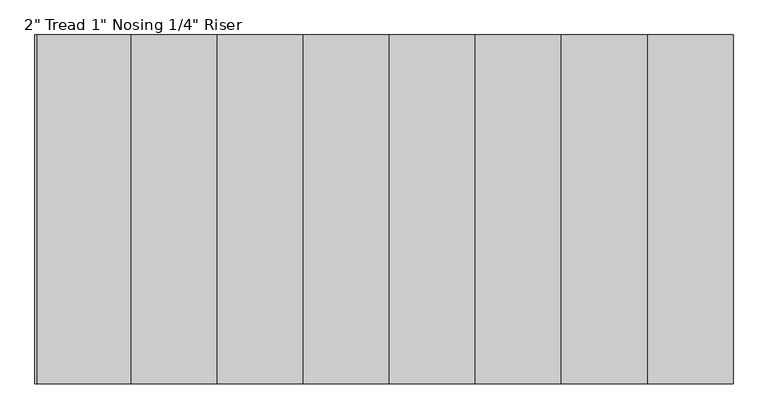
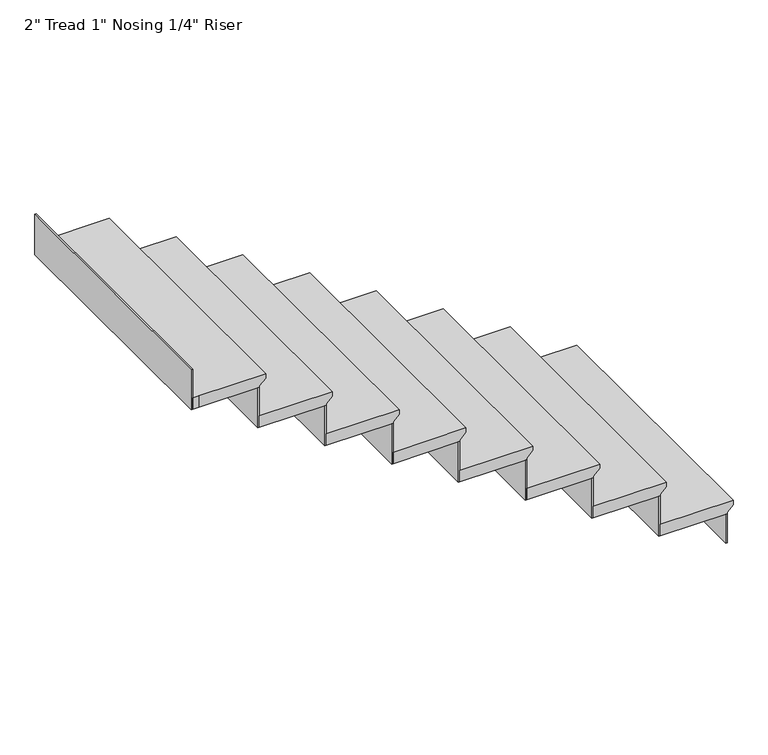
"""IFC4 building model written with IfcOpenShell, lengths in millimetres: stair flight geometry."""

from ifc_helpers import new_model, si_unit, origin, place, context, project, spatial, faceted_brep, source, transform, mapped, element, save


def stair_flight_1352b5f3(model_context):
    return source(origin(), model_context, "Body", "Brep", [
        faceted_brep([(-7986.2683044, -2706.1923176, 158.75), (-7986.2683044, -2706.1923176, 177.8), (-7986.2683044, -3838.3891189, 177.8), (-7986.2683044, -3838.3891189, 158.75), (-8011.6683044, -2706.1923176, 133.35), (-8011.6683044, -3838.3891189, 133.35), (-8291.0683044, -2706.1923176, 177.8), (-8291.0683044, -3838.3891189, 177.8), (-8011.6683044, -3838.3891189, 127.0), (-8291.0683044, -3838.3891189, 127.0), (-8291.0683044, -2706.1923176, 127.0), (-8011.6683044, -2706.1923176, 127.0)], [[[0, 1, 2, 3]], [[4, 0, 3, 5]], [[2, 1, 6, 7]], [[8, 9, 10, 11]], [[2, 7, 9, 8, 5, 3]], [[8, 11, 4, 5]], [[6, 1, 0, 4, 11, 10]], [[7, 6, 10, 9]]]),
        faceted_brep([(-8011.6683044, -2706.1923176, 127.0), (-8011.6683044, -2706.1923176, 0.0), (-8018.0183044, -2706.1923176, 0.0), (-8018.0183044, -2706.1923176, 127.0), (-8011.6683044, -3838.3891189, 127.0), (-8018.0183044, -3838.3891189, 127.0), (-8018.0183044, -3838.3891189, 0.0), (-8011.6683044, -3838.3891189, 0.0)], [[[0, 1, 2, 3]], [[4, 5, 6, 7]], [[1, 0, 4, 7]], [[2, 1, 7, 6]], [[3, 2, 6, 5]], [[0, 3, 5, 4]]]),
        faceted_brep([(-8291.0683044, -2706.1923176, 304.8), (-8291.0683044, -2706.1923176, 127.0), (-8297.4183044, -2706.1923176, 127.0), (-8297.4183044, -2706.1923176, 304.8), (-8291.0683044, -3838.3891189, 304.8), (-8297.4183044, -3838.3891189, 304.8), (-8297.4183044, -3838.3891189, 127.0), (-8291.0683044, -3838.3891189, 127.0)], [[[0, 1, 2, 3]], [[4, 5, 6, 7]], [[1, 0, 4, 7]], [[2, 1, 7, 6]], [[3, 2, 6, 5]], [[0, 3, 5, 4]]]),
        faceted_brep([(-8265.6683044, -3838.3891189, 355.6), (-8265.6683044, -2706.1923176, 355.6), (-8570.4683044, -2706.1923176, 355.6), (-8570.4683044, -3838.3891189, 355.6), (-8291.0683044, -3838.3891189, 304.8), (-8570.4683044, -3838.3891189, 304.8), (-8570.4683044, -2706.1923176, 304.8), (-8291.0683044, -2706.1923176, 304.8), (-8291.0683044, -3838.3891189, 311.15), (-8265.6683044, -3838.3891189, 336.55), (-8291.0683044, -2706.1923176, 311.15), (-8265.6683044, -2706.1923176, 336.55)], [[[0, 1, 2, 3]], [[4, 5, 6, 7]], [[0, 3, 5, 4, 8, 9]], [[4, 7, 10, 8]], [[2, 1, 11, 10, 7, 6]], [[3, 2, 6, 5]], [[11, 1, 0, 9]], [[10, 11, 9, 8]]]),
        faceted_brep([(-8570.4683044, -2706.1923176, 482.6), (-8570.4683044, -2706.1923176, 304.8), (-8576.8183044, -2706.1923176, 304.8), (-8576.8183044, -2706.1923176, 482.6), (-8570.4683044, -3838.3891189, 482.6), (-8576.8183044, -3838.3891189, 482.6), (-8576.8183044, -3838.3891189, 304.8), (-8570.4683044, -3838.3891189, 304.8)], [[[0, 1, 2, 3]], [[4, 5, 6, 7]], [[1, 0, 4, 7]], [[2, 1, 7, 6]], [[3, 2, 6, 5]], [[0, 3, 5, 4]]]),
        faceted_brep([(-8545.0683044, -3838.3891189, 533.4), (-8545.0683044, -2706.1923176, 533.4), (-8849.8683044, -2706.1923176, 533.4), (-8849.8683044, -3838.3891189, 533.4), (-8570.4683044, -3838.3891189, 482.6), (-8849.8683044, -3838.3891189, 482.6), (-8849.8683044, -2706.1923176, 482.6), (-8570.4683044, -2706.1923176, 482.6), (-8570.4683044, -3838.3891189, 488.95), (-8545.0683044, -3838.3891189, 514.35), (-8570.4683044, -2706.1923176, 488.95), (-8545.0683044, -2706.1923176, 514.35)], [[[0, 1, 2, 3]], [[4, 5, 6, 7]], [[0, 3, 5, 4, 8, 9]], [[4, 7, 10, 8]], [[2, 1, 11, 10, 7, 6]], [[3, 2, 6, 5]], [[11, 1, 0, 9]], [[10, 11, 9, 8]]]),
        faceted_brep([(-8849.8683044, -2706.1923176, 660.4), (-8849.8683044, -2706.1923176, 482.6), (-8856.2183044, -2706.1923176, 482.6), (-8856.2183044, -2706.1923176, 660.4), (-8849.8683044, -3838.3891189, 660.4), (-8856.2183044, -3838.3891189, 660.4), (-8856.2183044, -3838.3891189, 482.6), (-8849.8683044, -3838.3891189, 482.6)], [[[0, 1, 2, 3]], [[4, 5, 6, 7]], [[1, 0, 4, 7]], [[2, 1, 7, 6]], [[3, 2, 6, 5]], [[0, 3, 5, 4]]]),
        faceted_brep([(-8824.4683044, -3838.3891189, 711.2), (-8824.4683044, -2706.1923176, 711.2), (-9129.2683044, -2706.1923176, 711.2), (-9129.2683044, -3838.3891189, 711.2), (-8849.8683044, -3838.3891189, 660.4), (-9129.2683044, -3838.3891189, 660.4), (-9129.2683044, -2706.1923176, 660.4), (-8849.8683044, -2706.1923176, 660.4), (-8849.8683044, -3838.3891189, 666.75), (-8824.4683044, -3838.3891189, 692.15), (-8849.8683044, -2706.1923176, 666.75), (-8824.4683044, -2706.1923176, 692.15)], [[[0, 1, 2, 3]], [[4, 5, 6, 7]], [[0, 3, 5, 4, 8, 9]], [[4, 7, 10, 8]], [[2, 1, 11, 10, 7, 6]], [[3, 2, 6, 5]], [[11, 1, 0, 9]], [[10, 11, 9, 8]]]),
        faceted_brep([(-9129.2683044, -2706.1923176, 838.2), (-9129.2683044, -2706.1923176, 660.4), (-9135.6183044, -2706.1923176, 660.4), (-9135.6183044, -2706.1923176, 838.2), (-9129.2683044, -3838.3891189, 838.2), (-9135.6183044, -3838.3891189, 838.2), (-9135.6183044, -3838.3891189, 660.4), (-9129.2683044, -3838.3891189, 660.4)], [[[0, 1, 2, 3]], [[4, 5, 6, 7]], [[1, 0, 4, 7]], [[2, 1, 7, 6]], [[3, 2, 6, 5]], [[0, 3, 5, 4]]]),
        faceted_brep([(-9103.8683044, -3838.3891189, 889.0), (-9103.8683044, -2706.1923176, 889.0), (-9408.6683044, -2706.1923176, 889.0), (-9408.6683044, -3838.3891189, 889.0), (-9129.2683044, -3838.3891189, 838.2), (-9408.6683044, -3838.3891189, 838.2), (-9408.6683044, -2706.1923176, 838.2), (-9129.2683044, -2706.1923176, 838.2), (-9129.2683044, -3838.3891189, 844.55), (-9103.8683044, -3838.3891189, 869.95), (-9129.2683044, -2706.1923176, 844.55), (-9103.8683044, -2706.1923176, 869.95)], [[[0, 1, 2, 3]], [[4, 5, 6, 7]], [[0, 3, 5, 4, 8, 9]], [[4, 7, 10, 8]], [[2, 1, 11, 10, 7, 6]], [[3, 2, 6, 5]], [[11, 1, 0, 9]], [[10, 11, 9, 8]]]),
        faceted_brep([(-9408.6683044, -2706.1923176, 1016.0), (-9408.6683044, -2706.1923176, 838.2), (-9415.0183044, -2706.1923176, 838.2), (-9415.0183044, -2706.1923176, 1016.0), (-9408.6683044, -3838.3891189, 1016.0), (-9415.0183044, -3838.3891189, 1016.0), (-9415.0183044, -3838.3891189, 838.2), (-9408.6683044, -3838.3891189, 838.2)], [[[0, 1, 2, 3]], [[4, 5, 6, 7]], [[1, 0, 4, 7]], [[2, 1, 7, 6]], [[3, 2, 6, 5]], [[0, 3, 5, 4]]]),
        faceted_brep([(-9383.2683044, -3838.3891189, 1066.8), (-9383.2683044, -2706.1923176, 1066.8), (-9688.0683044, -2706.1923176, 1066.8), (-9688.0683044, -3838.3891189, 1066.8), (-9408.6683044, -3838.3891189, 1016.0), (-9688.0683044, -3838.3891189, 1016.0), (-9688.0683044, -2706.1923176, 1016.0), (-9408.6683044, -2706.1923176, 1016.0), (-9408.6683044, -3838.3891189, 1022.35), (-9383.2683044, -3838.3891189, 1047.75), (-9408.6683044, -2706.1923176, 1022.35), (-9383.2683044, -2706.1923176, 1047.75)], [[[0, 1, 2, 3]], [[4, 5, 6, 7]], [[0, 3, 5, 4, 8, 9]], [[4, 7, 10, 8]], [[2, 1, 11, 10, 7, 6]], [[3, 2, 6, 5]], [[11, 1, 0, 9]], [[10, 11, 9, 8]]]),
        faceted_brep([(-9688.0683044, -2706.1923176, 1193.8), (-9688.0683044, -2706.1923176, 1016.0), (-9694.4183044, -2706.1923176, 1016.0), (-9694.4183044, -2706.1923176, 1193.8), (-9688.0683044, -3838.3891189, 1193.8), (-9694.4183044, -3838.3891189, 1193.8), (-9694.4183044, -3838.3891189, 1016.0), (-9688.0683044, -3838.3891189, 1016.0)], [[[0, 1, 2, 3]], [[4, 5, 6, 7]], [[1, 0, 4, 7]], [[2, 1, 7, 6]], [[3, 2, 6, 5]], [[0, 3, 5, 4]]]),
        faceted_brep([(-9662.6683044, -3838.3891189, 1244.6), (-9662.6683044, -2706.1923176, 1244.6), (-9967.4683044, -2706.1923176, 1244.6), (-9967.4683044, -3838.3891189, 1244.6), (-9688.0683044, -3838.3891189, 1193.8), (-9967.4683044, -3838.3891189, 1193.8), (-9967.4683044, -2706.1923176, 1193.8), (-9688.0683044, -2706.1923176, 1193.8), (-9688.0683044, -3838.3891189, 1200.15), (-9662.6683044, -3838.3891189, 1225.55), (-9688.0683044, -2706.1923176, 1200.15), (-9662.6683044, -2706.1923176, 1225.55)], [[[0, 1, 2, 3]], [[4, 5, 6, 7]], [[0, 3, 5, 4, 8, 9]], [[4, 7, 10, 8]], [[2, 1, 11, 10, 7, 6]], [[3, 2, 6, 5]], [[11, 1, 0, 9]], [[10, 11, 9, 8]]]),
        faceted_brep([(-10246.8683044, -2706.1923176, 1549.4), (-10246.8683044, -2706.1923176, 1371.6), (-10253.2183044, -2706.1923176, 1371.6), (-10253.2183044, -2706.1923176, 1549.4), (-10246.8683044, -3838.3891189, 1549.4), (-10253.2183044, -3838.3891189, 1549.4), (-10253.2183044, -3838.3891189, 1371.6), (-10246.8683044, -3838.3891189, 1371.6)], [[[0, 1, 2, 3]], [[4, 5, 6, 7]], [[1, 0, 4, 7]], [[2, 1, 7, 6]], [[3, 2, 6, 5]], [[0, 3, 5, 4]]]),
        faceted_brep([(-9967.4683044, -2706.1923176, 1371.6), (-9967.4683044, -2706.1923176, 1193.8), (-9973.8183044, -2706.1923176, 1193.8), (-9973.8183044, -2706.1923176, 1371.6), (-9967.4683044, -3838.3891189, 1371.6), (-9973.8183044, -3838.3891189, 1371.6), (-9973.8183044, -3838.3891189, 1193.8), (-9967.4683044, -3838.3891189, 1193.8)], [[[0, 1, 2, 3]], [[4, 5, 6, 7]], [[1, 0, 4, 7]], [[2, 1, 7, 6]], [[3, 2, 6, 5]], [[0, 3, 5, 4]]]),
        faceted_brep([(-10246.8683044, -3838.3891189, 1422.4), (-10221.4683044, -3838.3891189, 1422.4), (-9942.0683044, -3838.3891189, 1422.4), (-9942.0683044, -2706.1923176, 1422.4), (-10246.8683044, -2706.1923176, 1422.4), (-10221.4683044, -3838.3891189, 1371.6), (-10246.8683044, -3838.3891189, 1371.6), (-10246.8683044, -2706.1923176, 1371.6), (-9967.4683044, -2706.1923176, 1371.6), (-9967.4683044, -3838.3891189, 1371.6), (-9967.4683044, -3838.3891189, 1377.95), (-9942.0683044, -3838.3891189, 1403.35), (-9967.4683044, -2706.1923176, 1377.95), (-9942.0683044, -2706.1923176, 1403.35)], [[[0, 1, 2, 3, 4]], [[5, 6, 7, 8, 9]], [[1, 0, 6, 5]], [[2, 1, 5, 9, 10, 11]], [[9, 8, 12, 10]], [[4, 3, 13, 12, 8, 7]], [[0, 4, 7, 6]], [[13, 3, 2, 11]], [[12, 13, 11, 10]]]),
    ])


if __name__ == "__main__":
    model = new_model("IFC4")
    model_context = context("Model", 3, world=origin())
    ifc_project = project(units=[si_unit("LENGTHUNIT", "METRE", prefix="MILLI")], contexts=[model_context])
    site = spatial("IfcSite", under=ifc_project)
    building = spatial("IfcBuilding", under=site)
    placement = place(None, origin())
    stair_flight_shape = stair_flight_1352b5f3(model_context)
    element("IfcStairFlight", 1, ObjectType="2\" Tread 1\" Nosing 1/4\" Riser", at=placement, inside=building, context=model_context, shape_type="MappedRepresentation", body=[
        mapped(stair_flight_shape, transform((0.0, 0.0, 0.0), x_axis=(1.0, 0.0, 0.0), y_axis=(0.0, 1.0, 0.0), z_axis=(0.0, 0.0, 1.0))),
    ])
    save(model, "model.ifc")
